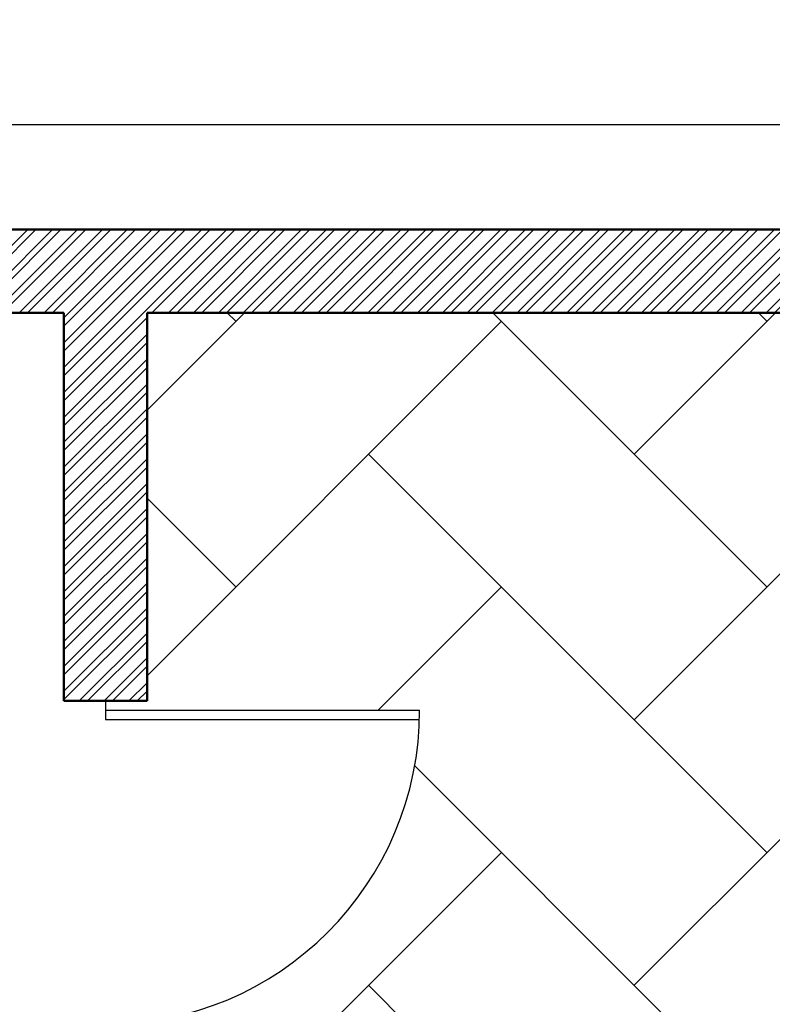
# Model space of a CAD drawing. Units: inches. Extents: x 3590 to 5167, y 65 to 1917.
# Tile 69 of 100: x 4919 to 5001, y 1722 to 1829. Entities that reach past the tile are written whole.
import ezdxf

# ---------------------------------------------------------------- set-up
doc = ezdxf.new("R2010")
doc.units = ezdxf.units.IN
for name, color, linetype, lineweight in [('A-ANNO-DIMS', 2, 'Continuous', 18), ('A-DOOR', 3, 'Continuous', 25), ('A-FLOR-PATT', 8, 'Continuous', 13), ('A-WALL', 7, 'Continuous', 50), ('A-WALL-PATT', 251, 'Continuous', 13)]:
    doc.layers.add(name, color=color, linetype=linetype, lineweight=lineweight)
doc.styles.get("Standard").update_dxf_attribs({"font": 'arial.ttf'})
doc.dimstyles.new('ISO-25', dxfattribs={"dimtxt": 9, "dimasz": 2.5, "dimexe": 1.25, "dimexo": 0.625, "dimtad": 1, "dimdec": 1, "dimlunit": 3, "dimtxsty": 'Standard', "dimcen": 2.5, "dimadec": 0, "dimazin": 0, "dimtfac": 1, "dimtdec": 1, "dimtmove": 0, "dimatfit": 3, "dimfxl": 1, "dimarcsym": 0})

# ---------------------------------------------------------------- blocks, each defined once
blk = doc.blocks.new('*D101')
at = {"layer": 'A-ANNO-DIMS', "color": 0, "lineweight": -2, "transparency": 16777216}
for p, q in [((4420.27, 1806.62), (4420.27, 1818.61)), ((5080.27, 1806.62), (5080.27, 1818.61)), ((4422.77, 1817.36), (5077.77, 1817.36))]:
    blk.add_line(p, q, dxfattribs=at)
at = {"layer": 'A-ANNO-DIMS', "color": 0, "transparency": 16777216}
for points in [[(4422.77, 1817.78), (4422.77, 1816.95), (4420.27, 1817.36)], [(5077.77, 1817.78), (5077.77, 1816.95), (5080.27, 1817.36)]]:
    blk.add_solid(points, dxfattribs=at)
at = {"layer": 'Defpoints', "color": 0, "transparency": 16777216}
for p in [(5080.27, 1817.36), (4420.27, 1806), (5080.27, 1806)]:
    blk.add_point(p, dxfattribs=at)
at = {"layer": 'A-ANNO-DIMS', "color": 0, "transparency": 16777216, "insert": (4750.27, 1822.57), "char_height": 9, "attachment_point": 5}
blk.add_mtext("55'", dxfattribs=at)
blk = doc.blocks.new('D1')
for p, q in [((1, 0), (1, 34)), ((2, 0), (2, 33.99)), ((0, 0), (2, 0)), ((35, 0), (36, 0))]:
    blk.add_line(p, q)
at = {"ltscale": 0.5}
blk.add_arc((1, 0), 34, 0, 90, dxfattribs=at)

msp = doc.modelspace()

# ---------------------------------------------------------------- hatches: boundary and pattern name
at = {"layer": 'A-FLOR-PATT', "transparency": 33554687}
h = msp.add_hatch(dxfattribs=at)
h.set_pattern_fill('AR-HBONE', color=256, scale=0.2)
h.set_pattern_definition([(45, (-588.972, 0), (0, 28.73682), [60.96, -20.32]), (135, (-574.604, 14.368), (3e-15, 28.73682), [60.96, -20.32])])
h.paths.add_polyline_path([(5071.27, 1797), (4933.27, 1797), (4933.27, 1754), (4962.77, 1754, -0.414214), (4928.77, 1720), (4933.27, 1719), (4933.27, 1335), (5071.27, 1335)])
h.paths.add_polyline_path([(4951.78, 1521.08), (4951.72, 1521.04), (4951.56, 1520.9)], flags=16)
h.paths.add_polyline_path([(4952.27, 1521.38), (4952.2, 1521.37), (4952.2, 1521.36)], flags=0)
h.paths.add_polyline_path([(4967.05, 1529.73), (4965.23, 1528.69), (4963.41, 1527.71), (4961.76, 1526.85), (4963.59, 1527.45), (4964.04, 1527.48), (4962.98, 1527.25), (4961.76, 1526.85), (4959.79, 1525.83), (4958, 1524.89), (4956.24, 1523.93), (4954.5, 1522.92), (4954.13, 1522.68), (4953.36, 1522), (4953.37, 1522), (4953.61, 1522.06), (4955.11, 1522.76), (4956.92, 1523.43), (4958.68, 1523.92), (4960.36, 1524.2), (4961.94, 1524.29), (4964.17, 1524.11), (4965.96, 1523.31), (4963.86, 1522.98), (4965.19, 1522.5), (4963.37, 1522.5), (4961.55, 1522.49), (4959.76, 1522.46), (4958.3, 1522.42), (4957.97, 1522.39), (4956.31, 1522.23), (4954.72, 1522.07), (4953.25, 1521.9), (4953.53, 1521.62), (4954.33, 1521.38), (4956.24, 1521.23), (4958.04, 1520.93), (4959.68, 1520.48), (4961.16, 1519.9), (4963.11, 1518.8), (4964.39, 1517.33), (4962.97, 1517.73), (4964.56, 1516.66), (4965.41, 1515.71), (4963.51, 1516.32), (4961.68, 1517.01), (4959.93, 1517.74), (4958.28, 1518.53), (4956.73, 1519.34), (4955.3, 1520.17), (4954.67, 1520.57), (4954.51, 1520.63), (4955.66, 1519.32), (4956.7, 1517.98), (4957.64, 1516.65), (4958.49, 1515.33), (4959.55, 1513.52), (4960.44, 1511.77), (4958.84, 1513.62), (4957.45, 1515.32), (4955.82, 1517.46), (4956.67, 1515.45), (4957.11, 1513.92), (4957.45, 1511.71), (4957.08, 1509.79), (4956.54, 1511.11), (4955.99, 1512.57), (4955.44, 1514.13), (4954.9, 1515.74), (4954.36, 1517.36), (4953.82, 1518.94), (4953.3, 1520.45), (4953.06, 1521.12), (4952.97, 1521.15), (4952.95, 1521.09), (4952.73, 1520.2), (4953.37, 1518.02), (4953.76, 1516.37), (4954.05, 1514.77), (4954.26, 1513.22), (4954.47, 1511.13), (4954.5, 1510.4), (4954.41, 1511.76), (4954.26, 1513.22), (4954.05, 1514.77), (4953.76, 1516.37), (4953.37, 1518.02), (4952.88, 1519.7), (4952.72, 1520.14), (4952.53, 1519.06), (4952.37, 1517.79), (4952.22, 1516.31), (4952.05, 1514.6), (4951.83, 1512.63), (4951.56, 1510.36), (4951.2, 1512.17), (4950.85, 1514.34), (4950.99, 1516.38), (4951.66, 1518.29), (4952.59, 1520.48), (4952.36, 1521.13), (4951.86, 1520.33), (4950.84, 1518.91), (4949.78, 1517.59), (4948.92, 1516.62), (4948.11, 1515.26), (4947.09, 1513.55), (4945.89, 1511.61), (4946.33, 1513.4), (4946.56, 1514.25), (4945.53, 1513.33), (4944.58, 1512.53), (4946.02, 1514.51), (4947.2, 1516.05), (4947.89, 1517.31), (4949.31, 1518.76), (4950.41, 1519.77), (4950.45, 1519.81), (4952.27, 1521.38), (4951.64, 1521.49), (4950.4, 1521.18), (4948.04, 1520.36), (4946.12, 1519.45), (4944.57, 1518.47), (4943.35, 1517.44), (4942, 1515.92), (4941.66, 1515.27), (4942.81, 1516.99), (4944.57, 1518.47), (4946.12, 1519.45), (4948.04, 1520.36), (4950.4, 1521.18), (4951.64, 1521.49), (4949.65, 1521.87), (4948.6, 1521.76), (4947.13, 1521.57), (4945.42, 1521.35), (4943.45, 1521.1), (4941.18, 1520.86), (4942.86, 1521.61), (4943.87, 1522.03), (4942.95, 1521.91), (4941.41, 1521.49), (4939.54, 1520.67), (4938.97, 1520.23), (4940.73, 1521.3), (4942.95, 1521.91), (4943.7, 1522.01), (4945.89, 1522.7), (4947.56, 1522.71), (4948.92, 1522.57), (4951.13, 1522.18), (4950.97, 1522.3), (4948.13, 1523.01), (4946.03, 1523.71), (4944.23, 1524.52), (4942.71, 1525.46), (4941.44, 1526.54), (4940.43, 1527.76), (4939.65, 1529.14), (4941.42, 1528.12), (4943.15, 1527.13), (4944.84, 1526.17), (4946.51, 1525.25), (4948.18, 1524.36), (4948.36, 1524.26), (4946.48, 1526.04), (4945.18, 1527.54), (4944.19, 1529.03), (4943.5, 1530.54), (4943.28, 1531.36), (4942.5, 1531.92), (4943.11, 1531.76), (4942.96, 1533.66), (4944.14, 1531.99), (4944.61, 1531.32), (4946.2, 1530.46), (4947.49, 1529.51), (4948.79, 1528.23), (4950.37, 1526.24), (4949.49, 1528.16), (4948.85, 1530.12), (4948.49, 1532.04), (4948.38, 1533.92), (4948.5, 1535.76), (4948.83, 1537.57), (4949.42, 1535.57), (4949.96, 1533.57), (4950.46, 1531.59), (4950.96, 1529.62), (4951.39, 1527.95), (4951.72, 1530.69), (4952.2, 1532.58), (4952.89, 1534.33), (4953.77, 1535.95), (4954.83, 1537.46), (4954.52, 1535.39), (4954.27, 1533.94), (4955.58, 1535.66), (4956.75, 1536.74), (4956.16, 1534.78), (4955.59, 1532.87), (4955.04, 1531.01), (4954.52, 1529.17), (4954.04, 1527.34), (4953.64, 1525.73), (4953.61, 1525.59), (4953.4, 1524.17), (4953.38, 1524.01), (4954.07, 1525.48), (4954.91, 1527.02), (4956.14, 1528.89), (4957.85, 1530.58), (4959.38, 1531.54), (4958.26, 1530.1), (4957.14, 1528.66), (4956.07, 1527.24), (4955.06, 1525.87), (4954.14, 1524.57), (4953.35, 1523.37), (4953.31, 1523.3), (4953.27, 1522.92), (4953.26, 1522.38), (4954.1, 1523.37), (4954.63, 1524.28), (4955.96, 1526.36), (4957.23, 1528.13), (4958.42, 1529.61), (4960.04, 1531.37), (4961.37, 1532.38), (4962.1, 1532.77), (4961.07, 1531.06), (4959.99, 1529.44), (4958.87, 1527.91), (4958.15, 1527.01), (4959.8, 1528), (4961.59, 1528.79), (4963.39, 1529.33), (4965.21, 1529.63)], flags=16)
h.paths.add_polyline_path([(4962.94, 1523.18), (4961.11, 1523.42), (4960.39, 1523.36), (4962.35, 1523.33)], flags=0)
h.paths.add_polyline_path([(5049.54, 1584.55), (5049.48, 1584.51), (5049.32, 1584.37)], flags=16)
h.paths.add_polyline_path([(5050.03, 1584.85), (5049.96, 1584.85), (5049.96, 1584.83)], flags=0)
h.paths.add_polyline_path([(5042.33, 1581.95), (5043.88, 1582.93), (5045.81, 1583.83), (5048.16, 1584.65), (5049.41, 1584.97), (5047.41, 1585.34), (5046.36, 1585.23), (5044.89, 1585.04), (5043.18, 1584.82), (5041.21, 1584.58), (5038.94, 1584.33), (5040.62, 1585.09), (5041.63, 1585.5), (5040.71, 1585.38), (5039.17, 1584.96), (5037.3, 1584.14), (5036.73, 1583.7), (5038.49, 1584.77), (5040.71, 1585.38), (5041.46, 1585.48), (5043.66, 1586.17), (5045.33, 1586.19), (5046.68, 1586.04), (5048.89, 1585.66), (5048.73, 1585.77), (5045.89, 1586.48), (5043.8, 1587.18), (5041.99, 1588), (5040.47, 1588.94), (5039.21, 1590.01), (5038.19, 1591.23), (5037.41, 1592.62), (5039.18, 1591.6), (5040.91, 1590.61), (5042.6, 1589.65), (5044.28, 1588.72), (5045.94, 1587.83), (5046.13, 1587.74), (5044.24, 1589.52), (5042.94, 1591.01), (5041.95, 1592.51), (5041.26, 1594.01), (5041.04, 1594.83), (5040.26, 1595.39), (5040.87, 1595.24), (5040.72, 1597.13), (5041.9, 1595.46), (5042.37, 1594.8), (5043.96, 1593.94), (5045.25, 1592.98), (5046.55, 1591.7), (5048.13, 1589.71), (5047.25, 1591.63), (5046.61, 1593.6), (5046.25, 1595.52), (5046.14, 1597.39), (5046.26, 1599.23), (5046.59, 1601.05), (5047.18, 1599.04), (5047.72, 1597.04), (5048.23, 1595.06), (5048.72, 1593.09), (5049.15, 1591.43), (5049.48, 1594.16), (5049.96, 1596.05), (5050.65, 1597.8), (5051.53, 1599.43), (5052.59, 1600.93), (5052.28, 1598.86), (5052.03, 1597.41), (5053.34, 1599.14), (5054.51, 1600.21), (5053.92, 1598.25), (5053.35, 1596.35), (5052.8, 1594.48), (5052.29, 1592.64), (5051.8, 1590.82), (5051.4, 1589.21), (5051.37, 1589.06), (5051.16, 1587.64), (5051.14, 1587.48), (5051.83, 1588.95), (5052.67, 1590.5), (5053.9, 1592.37), (5055.61, 1594.05), (5057.14, 1595.01), (5056.02, 1593.58), (5054.9, 1592.14), (5053.83, 1590.72), (5052.82, 1589.34), (5051.9, 1588.05), (5051.11, 1586.85), (5051.07, 1586.78), (5051.03, 1586.4), (5051.02, 1585.86), (5051.86, 1586.85), (5052.39, 1587.76), (5053.72, 1589.83), (5054.99, 1591.6), (5056.18, 1593.08), (5057.8, 1594.84), (5059.13, 1595.85), (5059.86, 1596.24), (5058.83, 1594.54), (5057.75, 1592.91), (5056.63, 1591.38), (5055.91, 1590.48), (5057.56, 1591.48), (5059.35, 1592.27), (5061.15, 1592.8), (5062.97, 1593.11), (5064.81, 1593.2), (5062.99, 1592.17), (5061.17, 1591.19), (5059.52, 1590.32), (5061.35, 1590.92), (5061.8, 1590.95), (5060.74, 1590.72), (5059.52, 1590.33), (5057.55, 1589.31), (5055.77, 1588.37), (5054, 1587.4), (5052.27, 1586.39), (5051.89, 1586.16), (5051.12, 1585.47), (5051.13, 1585.47), (5051.37, 1585.54), (5052.87, 1586.24), (5054.68, 1586.91), (5056.44, 1587.39), (5058.12, 1587.67), (5059.71, 1587.76), (5061.93, 1587.58), (5063.72, 1586.78), (5061.62, 1586.45), (5062.95, 1585.97), (5061.13, 1585.97), (5059.31, 1585.96), (5057.52, 1585.93), (5056.07, 1585.89), (5055.73, 1585.86), (5054.07, 1585.71), (5052.48, 1585.55), (5051.01, 1585.37), (5051.29, 1585.1), (5052.09, 1584.85), (5054, 1584.7), (5055.8, 1584.4), (5057.45, 1583.96), (5058.92, 1583.37), (5060.87, 1582.27), (5062.15, 1580.8), (5060.73, 1581.2), (5062.32, 1580.13), (5063.17, 1579.18), (5061.27, 1579.8), (5059.44, 1580.48), (5057.7, 1581.22), (5056.04, 1582), (5054.49, 1582.82), (5053.06, 1583.65), (5052.43, 1584.05), (5052.27, 1584.1), (5053.42, 1582.79), (5054.46, 1581.46), (5055.41, 1580.12), (5056.25, 1578.81), (5057.31, 1577), (5058.2, 1575.24), (5056.6, 1577.09), (5055.21, 1578.8), (5053.58, 1580.93), (5054.43, 1578.92), (5054.87, 1577.4), (5055.21, 1575.19), (5054.84, 1573.27), (5054.3, 1574.58), (5053.75, 1576.04), (5053.21, 1577.6), (5052.66, 1579.21), (5052.12, 1580.83), (5051.59, 1582.42), (5051.07, 1583.93), (5050.83, 1584.59), (5050.73, 1584.62), (5050.71, 1584.56), (5050.49, 1583.67), (5051.13, 1581.5), (5051.52, 1579.85), (5051.81, 1578.24), (5052.03, 1576.7), (5052.23, 1574.61), (5052.26, 1573.88), (5052.17, 1575.23), (5052.03, 1576.7), (5051.81, 1578.24), (5051.52, 1579.85), (5051.13, 1581.5), (5050.64, 1583.17), (5050.48, 1583.62), (5050.29, 1582.53), (5050.14, 1581.26), (5049.98, 1579.79), (5049.81, 1578.07), (5049.59, 1576.1), (5049.32, 1573.84), (5048.96, 1575.64), (5048.61, 1577.81), (5048.75, 1579.85), (5049.42, 1581.76), (5050.35, 1583.96), (5050.12, 1584.6), (5049.62, 1583.8), (5048.6, 1582.38), (5047.54, 1581.06), (5046.68, 1580.09), (5045.87, 1578.73), (5044.85, 1577.03), (5043.65, 1575.09), (5044.09, 1576.88), (5044.32, 1577.72), (5043.29, 1576.8), (5042.34, 1576.01), (5043.78, 1577.98), (5044.97, 1579.52), (5045.65, 1580.79), (5047.07, 1582.24), (5048.18, 1583.24), (5048.21, 1583.28), (5050.03, 1584.85), (5049.41, 1584.97), (5048.16, 1584.65), (5045.81, 1583.83), (5043.88, 1582.93), (5042.33, 1581.95), (5041.11, 1580.92), (5039.76, 1579.39), (5039.42, 1578.75), (5040.57, 1580.46)], flags=16)
h.paths.add_polyline_path([(4954.8, 1533.12), (4954.26, 1532.08), (4953.83, 1530.93), (4953.5, 1529.64), (4953.28, 1528.13), (4953.17, 1526.38), (4953.16, 1524.32), (4953.28, 1521.24), (4952.8, 1521.84), (4951.56, 1522), (4950.98, 1521.96), (4952.66, 1521.94), (4952.8, 1521.84), (4953.15, 1523.59), (4953.17, 1526.38), (4953.28, 1528.13), (4953.61, 1530.35), (4954.46, 1532.59)], flags=0)
h.paths.add_polyline_path([(5050.56, 1585.32), (5049.32, 1585.47), (5048.74, 1585.44), (5050.42, 1585.42), (5050.56, 1585.32), (5050.91, 1587.07), (5050.93, 1589.85), (5051.04, 1591.61), (5051.37, 1593.82), (5052.22, 1596.07), (5052.56, 1596.59), (5052.02, 1595.55), (5051.59, 1594.41), (5051.27, 1593.11), (5051.04, 1591.61), (5050.93, 1589.85), (5050.92, 1587.79), (5051.04, 1584.71)], flags=0)
h.paths.add_polyline_path([(5058.15, 1586.84), (5060.11, 1586.8), (5060.71, 1586.66), (5058.87, 1586.9)], flags=0)
h.paths.add_polyline_path([(5049.54, 1430.94), (5049.48, 1430.9), (5049.32, 1430.75)], flags=16)
h.paths.add_polyline_path([(5050.03, 1431.24), (5049.96, 1431.23), (5049.96, 1431.21)], flags=0)
h.paths.add_polyline_path([(5046.59, 1447.43), (5047.18, 1445.42), (5047.72, 1443.43), (5048.23, 1441.45), (5048.72, 1439.48), (5049.15, 1437.81), (5049.48, 1440.55), (5049.96, 1442.44), (5050.65, 1444.19), (5051.53, 1445.81), (5052.59, 1447.32), (5052.28, 1445.25), (5052.03, 1443.8), (5053.34, 1445.52), (5054.51, 1446.6), (5053.92, 1444.64), (5053.35, 1442.73), (5052.8, 1440.87), (5052.29, 1439.03), (5051.8, 1437.2), (5051.4, 1435.59), (5051.37, 1435.45), (5051.16, 1434.03), (5051.14, 1433.87), (5051.83, 1435.34), (5052.67, 1436.88), (5053.9, 1438.75), (5055.61, 1440.44), (5057.14, 1441.4), (5056.02, 1439.96), (5054.9, 1438.52), (5053.83, 1437.1), (5052.82, 1435.73), (5051.9, 1434.43), (5051.11, 1433.23), (5051.07, 1433.16), (5051.03, 1432.78), (5051.02, 1432.24), (5051.86, 1433.23), (5052.39, 1434.14), (5053.72, 1436.22), (5054.99, 1437.99), (5056.18, 1439.47), (5057.8, 1441.23), (5059.13, 1442.23), (5059.86, 1442.63), (5058.83, 1440.92), (5057.75, 1439.3), (5056.63, 1437.77), (5055.91, 1436.87), (5057.56, 1437.86), (5059.35, 1438.65), (5061.15, 1439.19), (5062.97, 1439.49), (5064.81, 1439.59), (5062.99, 1438.55), (5061.17, 1437.57), (5059.52, 1436.71), (5061.35, 1437.31), (5061.8, 1437.34), (5060.74, 1437.11), (5059.52, 1436.71), (5057.55, 1435.69), (5055.77, 1434.75), (5054, 1433.79), (5052.27, 1432.78), (5051.89, 1432.54), (5051.12, 1431.86), (5051.13, 1431.86), (5051.37, 1431.92), (5052.87, 1432.62), (5054.68, 1433.29), (5056.44, 1433.77), (5058.12, 1434.06), (5059.71, 1434.15), (5061.93, 1433.97), (5063.72, 1433.17), (5061.62, 1432.84), (5062.95, 1432.36), (5061.13, 1432.36), (5059.31, 1432.35), (5057.52, 1432.32), (5056.07, 1432.28), (5055.73, 1432.25), (5054.07, 1432.09), (5052.48, 1431.93), (5051.01, 1431.76), (5051.29, 1431.48), (5052.09, 1431.24), (5054, 1431.09), (5055.8, 1430.79), (5057.45, 1430.34), (5058.92, 1429.76), (5060.87, 1428.66), (5062.15, 1427.18), (5060.73, 1427.59), (5062.32, 1426.52), (5063.17, 1425.57), (5061.27, 1426.18), (5059.44, 1426.86), (5057.7, 1427.6), (5056.04, 1428.39), (5054.49, 1429.2), (5053.06, 1430.03), (5052.43, 1430.43), (5052.27, 1430.49), (5053.42, 1429.18), (5054.46, 1427.84), (5055.41, 1426.51), (5056.25, 1425.19), (5057.31, 1423.38), (5058.2, 1421.63), (5056.6, 1423.48), (5055.21, 1425.18), (5053.58, 1427.32), (5054.43, 1425.31), (5054.87, 1423.78), (5055.21, 1421.57), (5054.84, 1419.65), (5054.3, 1420.97), (5053.75, 1422.43), (5053.21, 1423.98), (5052.66, 1425.59), (5052.12, 1427.21), (5051.59, 1428.8), (5051.07, 1430.31), (5050.83, 1430.98), (5050.73, 1431.01), (5050.71, 1430.95), (5050.49, 1430.06), (5051.13, 1427.88), (5051.52, 1426.23), (5051.81, 1424.62), (5052.03, 1423.08), (5052.23, 1420.99), (5052.26, 1420.26), (5052.17, 1421.62), (5052.03, 1423.08), (5051.81, 1424.62), (5051.52, 1426.23), (5051.13, 1427.88), (5050.64, 1429.56), (5050.48, 1430), (5050.29, 1428.92), (5050.14, 1427.65), (5049.98, 1426.17), (5049.81, 1424.46), (5049.59, 1422.49), (5049.32, 1420.22), (5048.96, 1422.03), (5048.61, 1424.2), (5048.75, 1426.24), (5049.42, 1428.15), (5050.35, 1430.34), (5050.12, 1430.99), (5049.62, 1430.19), (5048.6, 1428.77), (5047.54, 1427.45), (5046.68, 1426.48), (5045.87, 1425.12), (5044.85, 1423.41), (5043.65, 1421.47), (5044.09, 1423.26), (5044.32, 1424.11), (5043.29, 1423.19), (5042.34, 1422.39), (5043.78, 1424.37), (5044.97, 1425.91), (5045.65, 1427.17), (5047.07, 1428.62), (5048.18, 1429.63), (5048.21, 1429.67), (5050.03, 1431.24), (5049.41, 1431.35), (5048.16, 1431.04), (5045.81, 1430.22), (5043.88, 1429.31), (5042.33, 1428.33), (5041.11, 1427.3), (5039.76, 1425.78), (5039.42, 1425.13), (5040.57, 1426.85), (5042.33, 1428.33), (5043.88, 1429.31), (5045.81, 1430.22), (5048.16, 1431.04), (5049.41, 1431.35), (5047.41, 1431.73), (5046.36, 1431.62), (5044.89, 1431.43), (5043.18, 1431.21), (5041.21, 1430.96), (5038.94, 1430.72), (5040.62, 1431.47), (5041.63, 1431.89), (5040.71, 1431.77), (5039.17, 1431.34), (5037.3, 1430.53), (5036.73, 1430.08), (5038.49, 1431.16), (5040.71, 1431.77), (5041.46, 1431.87), (5043.66, 1432.56), (5045.33, 1432.57), (5046.68, 1432.43), (5048.89, 1432.04), (5048.73, 1432.16), (5045.89, 1432.87), (5043.8, 1433.57), (5041.99, 1434.38), (5040.47, 1435.32), (5039.21, 1436.4), (5038.19, 1437.62), (5037.41, 1439), (5039.18, 1437.98), (5040.91, 1436.99), (5042.6, 1436.03), (5044.28, 1435.11), (5045.94, 1434.22), (5046.13, 1434.12), (5044.24, 1435.9), (5042.94, 1437.4), (5041.95, 1438.89), (5041.26, 1440.4), (5041.04, 1441.22), (5040.26, 1441.78), (5040.87, 1441.62), (5040.72, 1443.52), (5041.9, 1441.85), (5042.37, 1441.18), (5043.96, 1440.32), (5045.25, 1439.37), (5046.55, 1438.09), (5048.13, 1436.1), (5047.25, 1438.01), (5046.61, 1439.98), (5046.25, 1441.9), (5046.14, 1443.78), (5046.26, 1445.62)], flags=16)
h.paths.add_polyline_path([(5052.38, 1444.25), (5051.62, 1442.78), (5052.02, 1441.94), (5052.56, 1442.98)], flags=0)
h.paths.add_polyline_path([(5050.56, 1431.7), (5049.32, 1431.86), (5048.74, 1431.82), (5050.42, 1431.8)], flags=0)
h.paths.add_polyline_path([(5058.15, 1433.22), (5060.11, 1433.19), (5060.71, 1433.04), (5058.87, 1433.28)], flags=0)
h.paths.add_polyline_path([(5049.54, 1352.29), (5049.48, 1352.25), (5049.32, 1352.1)], flags=16)
h.paths.add_polyline_path([(5050.03, 1352.59), (5049.96, 1352.58), (5049.96, 1352.56)], flags=0)
h.paths.add_polyline_path([(5046.59, 1368.78), (5047.18, 1366.77), (5047.72, 1364.78), (5048.23, 1362.79), (5048.72, 1360.83), (5049.15, 1359.16), (5049.48, 1361.9), (5049.96, 1363.79), (5050.65, 1365.54), (5051.53, 1367.16), (5052.59, 1368.67), (5052.28, 1366.6), (5052.03, 1365.15), (5053.34, 1366.87), (5054.51, 1367.95), (5053.92, 1365.99), (5053.35, 1364.08), (5052.8, 1362.21), (5052.29, 1360.37), (5051.8, 1358.55), (5051.4, 1356.94), (5051.37, 1356.79), (5051.16, 1355.37), (5051.14, 1355.22), (5051.83, 1356.68), (5052.67, 1358.23), (5053.9, 1360.1), (5055.61, 1361.79), (5057.14, 1362.75), (5056.02, 1361.31), (5054.9, 1359.87), (5053.83, 1358.45), (5052.82, 1357.08), (5051.9, 1355.78), (5051.11, 1354.58), (5051.07, 1354.51), (5051.03, 1354.13), (5051.02, 1353.59), (5051.86, 1354.58), (5052.39, 1355.49), (5053.72, 1357.57), (5054.99, 1359.34), (5056.18, 1360.82), (5057.8, 1362.58), (5059.13, 1363.58), (5059.86, 1363.98), (5058.83, 1362.27), (5057.75, 1360.65), (5056.63, 1359.12), (5055.91, 1358.22), (5057.56, 1359.21), (5059.35, 1360), (5061.15, 1360.54), (5062.97, 1360.84), (5064.81, 1360.94), (5062.99, 1359.9), (5061.17, 1358.92), (5059.52, 1358.06), (5061.35, 1358.66), (5061.8, 1358.69), (5060.74, 1358.46), (5059.52, 1358.06), (5057.55, 1357.04), (5055.77, 1356.1), (5054, 1355.14), (5052.27, 1354.13), (5051.89, 1353.89), (5051.12, 1353.21), (5051.13, 1353.21), (5051.37, 1353.27), (5052.87, 1353.97), (5054.68, 1354.64), (5056.44, 1355.12), (5058.12, 1355.41), (5059.71, 1355.49), (5061.93, 1355.32), (5063.72, 1354.52), (5061.62, 1354.18), (5062.95, 1353.71), (5061.13, 1353.71), (5059.31, 1353.7), (5057.52, 1353.67), (5056.07, 1353.63), (5055.73, 1353.6), (5054.07, 1353.44), (5052.48, 1353.28), (5051.01, 1353.11), (5051.29, 1352.83), (5052.09, 1352.59), (5054, 1352.44), (5055.8, 1352.14), (5057.45, 1351.69), (5058.92, 1351.1), (5060.87, 1350.01), (5062.15, 1348.53), (5060.73, 1348.93), (5062.32, 1347.87), (5063.17, 1346.92), (5061.27, 1347.53), (5059.44, 1348.21), (5057.7, 1348.95), (5056.04, 1349.74), (5054.49, 1350.55), (5053.06, 1351.38), (5052.43, 1351.78), (5052.27, 1351.84), (5053.42, 1350.53), (5054.46, 1349.19), (5055.41, 1347.86), (5056.25, 1346.54), (5057.31, 1344.73), (5058.2, 1342.98), (5056.6, 1344.83), (5055.21, 1346.53), (5053.58, 1348.67), (5054.43, 1346.66), (5054.87, 1345.13), (5055.21, 1342.92), (5054.84, 1341), (5054.3, 1342.32), (5053.75, 1343.78), (5053.21, 1345.33), (5052.66, 1346.94), (5052.12, 1348.56), (5051.59, 1350.15), (5051.07, 1351.66), (5050.83, 1352.32), (5050.73, 1352.35), (5050.71, 1352.3), (5050.49, 1351.41), (5051.13, 1349.23), (5051.52, 1347.58), (5051.81, 1345.97), (5052.03, 1344.43), (5052.23, 1342.34), (5052.26, 1341.61), (5052.17, 1342.97), (5052.03, 1344.43), (5051.81, 1345.97), (5051.52, 1347.58), (5051.13, 1349.23), (5050.64, 1350.91), (5050.48, 1351.35), (5050.29, 1350.27), (5050.14, 1349), (5049.98, 1347.52), (5049.81, 1345.81), (5049.59, 1343.83), (5049.32, 1341.57), (5048.96, 1343.38), (5048.61, 1345.55), (5048.75, 1347.58), (5049.42, 1349.49), (5050.35, 1351.69), (5050.12, 1352.34), (5049.62, 1351.54), (5048.6, 1350.12), (5047.54, 1348.8), (5046.68, 1347.83), (5045.87, 1346.46), (5044.85, 1344.76), (5043.65, 1342.82), (5044.09, 1344.61), (5044.32, 1345.46), (5043.29, 1344.54), (5042.34, 1343.74), (5043.78, 1345.72), (5044.97, 1347.26), (5045.65, 1348.52), (5047.07, 1349.97), (5048.18, 1350.98), (5048.21, 1351.01), (5050.03, 1352.59), (5049.41, 1352.7), (5048.16, 1352.39), (5045.81, 1351.57), (5043.88, 1350.66), (5042.33, 1349.68), (5041.11, 1348.65), (5039.76, 1347.13), (5039.42, 1346.48), (5040.57, 1348.2), (5042.33, 1349.68), (5043.88, 1350.66), (5045.81, 1351.57), (5048.16, 1352.39), (5049.41, 1352.7), (5047.41, 1353.08), (5046.36, 1352.96), (5044.89, 1352.78), (5043.18, 1352.56), (5041.21, 1352.31), (5038.94, 1352.06), (5040.62, 1352.82), (5041.63, 1353.24), (5040.71, 1353.12), (5039.17, 1352.69), (5037.3, 1351.88), (5036.73, 1351.43), (5038.49, 1352.51), (5040.71, 1353.12), (5041.46, 1353.22), (5043.66, 1353.91), (5045.33, 1353.92), (5046.68, 1353.77), (5048.89, 1353.39), (5048.73, 1353.51), (5045.89, 1354.21), (5043.8, 1354.92), (5041.99, 1355.73), (5040.47, 1356.67), (5039.21, 1357.75), (5038.19, 1358.97), (5037.41, 1360.35), (5039.18, 1359.33), (5040.91, 1358.34), (5042.6, 1357.38), (5044.28, 1356.46), (5045.94, 1355.57), (5046.13, 1355.47), (5044.24, 1357.25), (5042.94, 1358.75), (5041.95, 1360.24), (5041.26, 1361.75), (5041.04, 1362.57), (5040.26, 1363.13), (5040.87, 1362.97), (5040.72, 1364.87), (5041.9, 1363.2), (5042.37, 1362.53), (5043.96, 1361.67), (5045.25, 1360.72), (5046.55, 1359.44), (5048.13, 1357.45), (5047.25, 1359.36), (5046.61, 1361.33), (5046.25, 1363.25), (5046.14, 1365.13), (5046.26, 1366.97)], flags=16)
h.paths.add_polyline_path([(5052.38, 1365.6), (5051.62, 1364.13), (5052.02, 1363.29), (5052.56, 1364.33)], flags=0)
h.paths.add_polyline_path([(4951.78, 1698.04), (4951.72, 1698), (4951.56, 1697.86)], flags=16)
h.paths.add_polyline_path([(4952.27, 1698.34), (4952.2, 1698.34), (4952.2, 1698.32)], flags=0)
h.paths.add_polyline_path([(4957.08, 1686.76), (4956.54, 1688.07), (4955.99, 1689.53), (4955.44, 1691.09), (4954.9, 1692.7), (4954.36, 1694.32), (4953.82, 1695.91), (4953.3, 1697.42), (4953.06, 1698.08), (4952.97, 1698.11), (4952.95, 1698.05), (4952.73, 1697.16), (4953.37, 1694.99), (4953.76, 1693.34), (4954.05, 1691.73), (4954.26, 1690.19), (4954.47, 1688.1), (4954.5, 1687.37), (4954.41, 1688.72), (4954.26, 1690.19), (4954.05, 1691.73), (4953.76, 1693.34), (4953.37, 1694.99), (4952.88, 1696.66), (4952.72, 1697.11), (4952.53, 1696.02), (4952.37, 1694.75), (4952.22, 1693.28), (4952.05, 1691.56), (4951.83, 1689.59), (4951.56, 1687.33), (4951.2, 1689.13), (4950.85, 1691.3), (4950.99, 1693.34), (4951.66, 1695.25), (4952.59, 1697.44), (4952.36, 1698.09), (4951.86, 1697.29), (4950.84, 1695.87), (4949.78, 1694.55), (4948.92, 1693.58), (4948.11, 1692.22), (4947.09, 1690.52), (4945.89, 1688.58), (4946.33, 1690.37), (4946.56, 1691.21), (4945.53, 1690.29), (4944.58, 1689.5), (4946.02, 1691.47), (4947.2, 1693.01), (4947.89, 1694.28), (4949.31, 1695.73), (4950.41, 1696.73), (4950.45, 1696.77), (4952.27, 1698.34), (4951.64, 1698.46), (4950.4, 1698.14), (4948.04, 1697.32), (4946.12, 1696.42), (4944.57, 1695.44), (4943.35, 1694.41), (4942, 1692.88), (4941.66, 1692.24), (4942.81, 1693.95), (4944.57, 1695.44), (4946.12, 1696.42), (4948.04, 1697.32), (4950.4, 1698.14), (4951.64, 1698.46), (4949.65, 1698.83), (4948.6, 1698.72), (4947.13, 1698.53), (4945.42, 1698.31), (4943.45, 1698.07), (4941.18, 1697.82), (4942.86, 1698.58), (4943.87, 1698.99), (4942.95, 1698.87), (4941.41, 1698.45), (4939.54, 1697.63), (4938.97, 1697.19), (4940.73, 1698.26), (4942.95, 1698.87), (4943.7, 1698.97), (4945.89, 1699.66), (4947.56, 1699.68), (4948.92, 1699.53), (4951.13, 1699.15), (4950.97, 1699.26), (4948.13, 1699.97), (4946.03, 1700.67), (4944.23, 1701.49), (4942.71, 1702.43), (4941.44, 1703.5), (4940.43, 1704.72), (4939.65, 1706.11), (4941.42, 1705.09), (4943.15, 1704.1), (4944.84, 1703.14), (4946.51, 1702.21), (4948.18, 1701.32), (4948.36, 1701.23), (4946.48, 1703.01), (4945.18, 1704.5), (4944.19, 1706), (4943.5, 1707.5), (4943.28, 1708.32), (4942.5, 1708.88), (4943.11, 1708.73), (4942.96, 1710.62), (4944.14, 1708.95), (4944.61, 1708.29), (4946.2, 1707.43), (4947.49, 1706.47), (4948.79, 1705.19), (4950.37, 1703.2), (4949.49, 1705.12), (4948.85, 1707.09), (4948.49, 1709.01), (4948.38, 1710.88), (4948.5, 1712.72), (4948.83, 1714.54), (4949.42, 1712.53), (4949.96, 1710.53), (4950.46, 1708.55), (4950.96, 1706.58), (4951.39, 1704.92), (4951.72, 1707.65), (4952.2, 1709.54), (4952.89, 1711.29), (4953.77, 1712.92), (4954.83, 1714.42), (4954.52, 1712.35), (4954.27, 1710.9), (4955.58, 1712.63), (4956.75, 1713.7), (4956.16, 1711.74), (4955.59, 1709.84), (4955.04, 1707.97), (4954.52, 1706.13), (4954.04, 1704.31), (4953.64, 1702.7), (4953.61, 1702.55), (4953.4, 1701.13), (4953.38, 1700.97), (4954.07, 1702.44), (4954.91, 1703.99), (4956.14, 1705.86), (4957.85, 1707.54), (4959.38, 1708.5), (4958.26, 1707.07), (4957.14, 1705.63), (4956.07, 1704.21), (4955.06, 1702.83), (4954.14, 1701.54), (4953.35, 1700.34), (4953.31, 1700.27), (4953.27, 1699.89), (4953.26, 1699.35), (4954.1, 1700.34), (4954.63, 1701.25), (4955.96, 1703.32), (4957.23, 1705.09), (4958.42, 1706.57), (4960.04, 1708.33), (4961.37, 1709.34), (4962.1, 1709.73), (4961.07, 1708.03), (4959.99, 1706.4), (4958.87, 1704.87), (4958.15, 1703.97), (4959.8, 1704.97), (4961.59, 1705.76), (4963.39, 1706.29), (4965.21, 1706.6), (4967.05, 1706.69), (4965.23, 1705.66), (4963.41, 1704.68), (4961.76, 1703.81), (4963.59, 1704.41), (4964.04, 1704.44), (4962.98, 1704.21), (4961.76, 1703.82), (4959.79, 1702.8), (4958, 1701.86), (4956.24, 1700.89), (4954.5, 1699.88), (4954.13, 1699.65), (4953.36, 1698.96), (4953.37, 1698.96), (4953.61, 1699.03), (4955.11, 1699.72), (4956.92, 1700.4), (4958.68, 1700.88), (4960.36, 1701.16), (4961.94, 1701.25), (4964.17, 1701.07), (4965.96, 1700.27), (4963.86, 1699.94), (4965.19, 1699.46), (4963.37, 1699.46), (4961.55, 1699.45), (4959.76, 1699.42), (4958.3, 1699.38), (4957.97, 1699.35), (4956.31, 1699.2), (4954.72, 1699.04), (4953.25, 1698.86), (4953.53, 1698.59), (4954.33, 1698.34), (4956.24, 1698.19), (4958.04, 1697.89), (4959.68, 1697.45), (4961.16, 1696.86), (4963.11, 1695.76), (4964.39, 1694.29), (4962.97, 1694.69), (4964.56, 1693.62), (4965.41, 1692.67), (4963.51, 1693.29), (4961.68, 1693.97), (4959.93, 1694.71), (4958.28, 1695.49), (4956.73, 1696.31), (4955.3, 1697.14), (4954.67, 1697.54), (4954.51, 1697.59), (4955.66, 1696.28), (4956.7, 1694.95), (4957.64, 1693.61), (4958.49, 1692.3), (4959.55, 1690.49), (4960.44, 1688.73), (4958.84, 1690.58), (4957.45, 1692.29), (4955.82, 1694.42), (4956.67, 1692.41), (4957.11, 1690.89), (4957.45, 1688.68)], flags=16)
h.paths.add_polyline_path([(5050.56, 1353.05), (5049.32, 1353.21), (5048.74, 1353.17), (5050.42, 1353.15)], flags=0)
h.paths.add_polyline_path([(4951.78, 1351.49), (4951.72, 1351.45), (4951.56, 1351.3)], flags=16)
h.paths.add_polyline_path([(4952.27, 1351.79), (4952.2, 1351.78), (4952.2, 1351.76)], flags=0)
h.paths.add_polyline_path([(4954.83, 1367.87), (4954.52, 1365.8), (4954.27, 1364.35), (4955.58, 1366.07), (4956.75, 1367.15), (4956.16, 1365.19), (4955.59, 1363.28), (4955.04, 1361.42), (4954.52, 1359.58), (4954.04, 1357.75), (4953.64, 1356.14), (4953.61, 1356), (4953.4, 1354.58), (4953.38, 1354.42), (4954.07, 1355.89), (4954.91, 1357.43), (4956.14, 1359.3), (4957.85, 1360.99), (4959.38, 1361.95), (4958.26, 1360.51), (4957.14, 1359.07), (4956.07, 1357.65), (4955.06, 1356.28), (4954.14, 1354.98), (4953.35, 1353.78), (4953.31, 1353.71), (4953.27, 1353.33), (4953.26, 1352.79), (4954.1, 1353.78), (4954.63, 1354.69), (4955.96, 1356.77), (4957.23, 1358.54), (4958.42, 1360.02), (4960.04, 1361.78), (4961.37, 1362.78), (4962.1, 1363.18), (4961.07, 1361.47), (4959.99, 1359.85), (4958.87, 1358.32), (4958.15, 1357.42), (4959.8, 1358.41), (4961.59, 1359.2), (4963.39, 1359.74), (4965.21, 1360.04), (4967.05, 1360.14), (4965.23, 1359.1), (4963.41, 1358.12), (4961.76, 1357.26), (4963.59, 1357.86), (4964.04, 1357.89), (4962.98, 1357.66), (4961.76, 1357.26), (4959.79, 1356.24), (4958, 1355.3), (4956.24, 1354.34), (4954.5, 1353.33), (4954.13, 1353.09), (4953.36, 1352.41), (4953.37, 1352.41), (4953.61, 1352.47), (4955.11, 1353.17), (4956.92, 1353.84), (4958.68, 1354.32), (4960.36, 1354.61), (4961.94, 1354.7), (4964.17, 1354.52), (4965.96, 1353.72), (4963.86, 1353.39), (4965.19, 1352.91), (4963.37, 1352.91), (4961.55, 1352.9), (4959.76, 1352.87), (4958.3, 1352.83), (4957.97, 1352.8), (4956.31, 1352.64), (4954.72, 1352.48), (4953.25, 1352.31), (4953.53, 1352.03), (4954.33, 1351.79), (4956.24, 1351.64), (4958.04, 1351.34), (4959.68, 1350.89), (4961.16, 1350.31), (4963.11, 1349.21), (4964.39, 1347.73), (4962.97, 1348.14), (4964.56, 1347.07), (4965.41, 1346.12), (4963.51, 1346.73), (4961.68, 1347.41), (4959.93, 1348.15), (4958.28, 1348.94), (4956.73, 1349.75), (4955.3, 1350.58), (4954.67, 1350.98), (4954.51, 1351.04), (4955.66, 1349.73), (4956.7, 1348.39), (4957.64, 1347.06), (4958.49, 1345.74), (4959.55, 1343.93), (4960.44, 1342.18), (4958.84, 1344.03), (4957.45, 1345.73), (4955.82, 1347.87), (4956.67, 1345.86), (4957.11, 1344.33), (4957.45, 1342.12), (4957.08, 1340.2), (4956.54, 1341.52), (4955.99, 1342.98), (4955.44, 1344.53), (4954.9, 1346.14), (4954.36, 1347.76), (4953.82, 1349.35), (4953.3, 1350.86), (4953.06, 1351.53), (4952.97, 1351.56), (4952.95, 1351.5), (4952.73, 1350.61), (4953.37, 1348.43), (4953.76, 1346.78), (4954.05, 1345.17), (4954.26, 1343.63), (4954.47, 1341.54), (4954.5, 1340.81), (4954.41, 1342.17), (4954.26, 1343.63), (4954.05, 1345.17), (4953.76, 1346.78), (4953.37, 1348.43), (4952.88, 1350.11), (4952.72, 1350.55), (4952.53, 1349.47), (4952.37, 1348.2), (4952.22, 1346.72), (4952.05, 1345.01), (4951.83, 1343.04), (4951.56, 1340.77), (4951.2, 1342.58), (4950.85, 1344.75), (4950.99, 1346.79), (4951.66, 1348.7), (4952.59, 1350.89), (4952.36, 1351.54), (4951.86, 1350.74), (4950.84, 1349.32), (4949.78, 1348), (4948.92, 1347.03), (4948.11, 1345.67), (4947.09, 1343.96), (4945.89, 1342.02), (4946.33, 1343.81), (4946.56, 1344.66), (4945.53, 1343.74), (4944.58, 1342.94), (4946.02, 1344.92), (4947.2, 1346.46), (4947.89, 1347.72), (4949.31, 1349.17), (4950.41, 1350.18), (4950.45, 1350.22), (4952.27, 1351.79), (4951.64, 1351.9), (4950.4, 1351.59), (4948.04, 1350.77), (4946.12, 1349.86), (4944.57, 1348.88), (4943.35, 1347.85), (4942, 1346.33), (4941.66, 1345.68), (4942.81, 1347.4), (4944.57, 1348.88), (4946.12, 1349.86), (4948.04, 1350.77), (4950.4, 1351.59), (4951.64, 1351.9), (4949.65, 1352.28), (4948.6, 1352.17), (4947.13, 1351.98), (4945.42, 1351.76), (4943.45, 1351.51), (4941.18, 1351.27), (4942.86, 1352.02), (4943.87, 1352.44), (4942.95, 1352.32), (4941.41, 1351.89), (4939.54, 1351.08), (4938.97, 1350.63), (4940.73, 1351.71), (4942.95, 1352.32), (4943.7, 1352.42), (4945.89, 1353.11), (4947.56, 1353.12), (4948.92, 1352.98), (4951.13, 1352.59), (4950.97, 1352.71), (4948.13, 1353.42), (4946.03, 1354.12), (4944.23, 1354.93), (4942.71, 1355.87), (4941.44, 1356.95), (4940.43, 1358.17), (4939.65, 1359.55), (4941.42, 1358.53), (4943.15, 1357.54), (4944.84, 1356.58), (4946.51, 1355.66), (4948.18, 1354.77), (4948.36, 1354.67), (4946.48, 1356.45), (4945.18, 1357.95), (4944.19, 1359.44), (4943.5, 1360.95), (4943.28, 1361.77), (4942.5, 1362.33), (4943.11, 1362.17), (4942.96, 1364.07), (4944.14, 1362.4), (4944.61, 1361.73), (4946.2, 1360.87), (4947.49, 1359.92), (4948.79, 1358.64), (4950.37, 1356.65), (4949.49, 1358.56), (4948.85, 1360.53), (4948.49, 1362.45), (4948.38, 1364.33), (4948.5, 1366.17), (4948.83, 1367.98), (4949.42, 1365.97), (4949.96, 1363.98), (4950.46, 1362), (4950.96, 1360.03), (4951.39, 1358.36), (4951.72, 1361.1), (4952.2, 1362.99), (4952.89, 1364.74), (4953.77, 1366.36)], flags=16)
h.paths.add_polyline_path([(4954.8, 1363.53), (4954.26, 1362.49), (4953.83, 1361.34), (4953.5, 1360.05), (4953.28, 1358.54), (4953.17, 1356.79), (4953.16, 1354.72), (4953.28, 1351.65), (4952.8, 1352.25), (4951.56, 1352.41), (4950.98, 1352.37), (4952.66, 1352.35), (4952.8, 1352.25), (4953.15, 1354), (4953.17, 1356.79), (4953.28, 1358.54), (4953.61, 1360.76), (4954.46, 1363)], flags=0)
h.paths.add_polyline_path([(4952.8, 1698.81), (4951.56, 1698.96), (4950.98, 1698.93), (4952.66, 1698.91), (4952.8, 1698.81), (4953.15, 1700.56), (4953.17, 1703.34), (4953.28, 1705.1), (4953.61, 1707.31), (4954.46, 1709.56), (4954.8, 1710.08), (4954.26, 1709.04), (4953.83, 1707.9), (4953.5, 1706.6), (4953.28, 1705.1), (4953.17, 1703.34), (4953.16, 1701.28), (4953.28, 1698.2)], flags=0)
h.paths.add_polyline_path([(4962.94, 1700.15), (4961.11, 1700.39), (4960.39, 1700.33), (4962.35, 1700.29)], flags=0)
h.paths.add_polyline_path([(5058.15, 1354.57), (5060.11, 1354.54), (5060.71, 1354.39), (5058.87, 1354.63)], flags=0)
h.paths.add_polyline_path([(4962.94, 1353.59), (4961.11, 1353.83), (4960.39, 1353.77), (4962.35, 1353.74)], flags=0)
h.paths.add_polyline_path([(5049.54, 1778.72), (5049.48, 1778.68), (5049.32, 1778.54)], flags=16)
h.paths.add_polyline_path([(5050.03, 1779.02), (5049.96, 1779.01), (5049.96, 1779)], flags=0)
h.paths.add_polyline_path([(5052.26, 1768.04), (5052.17, 1769.4), (5052.03, 1770.86), (5051.81, 1772.41), (5051.52, 1774.02), (5051.13, 1775.67), (5050.64, 1777.34), (5050.48, 1777.78), (5050.29, 1776.7), (5050.14, 1775.43), (5049.98, 1773.95), (5049.81, 1772.24), (5049.59, 1770.27), (5049.32, 1768.01), (5048.96, 1769.81), (5048.61, 1771.98), (5048.75, 1774.02), (5049.42, 1775.93), (5050.35, 1778.12), (5050.12, 1778.77), (5049.62, 1777.97), (5048.6, 1776.55), (5047.54, 1775.23), (5046.68, 1774.26), (5045.87, 1772.9), (5044.85, 1771.2), (5043.65, 1769.26), (5044.09, 1771.05), (5044.32, 1771.89), (5043.29, 1770.97), (5042.34, 1770.17), (5043.78, 1772.15), (5044.97, 1773.69), (5045.65, 1774.96), (5047.07, 1776.41), (5048.18, 1777.41), (5048.21, 1777.45), (5050.03, 1779.02), (5049.41, 1779.14), (5048.16, 1778.82), (5045.81, 1778), (5043.88, 1777.1), (5042.33, 1776.12), (5041.11, 1775.09), (5039.76, 1773.56), (5039.42, 1772.92), (5040.57, 1774.63), (5042.33, 1776.12), (5043.88, 1777.1), (5045.81, 1778), (5048.16, 1778.82), (5049.41, 1779.14), (5047.41, 1779.51), (5046.36, 1779.4), (5044.89, 1779.21), (5043.18, 1778.99), (5041.21, 1778.75), (5038.94, 1778.5), (5040.62, 1779.26), (5041.63, 1779.67), (5040.71, 1779.55), (5039.17, 1779.13), (5037.3, 1778.31), (5036.73, 1777.87), (5038.49, 1778.94), (5040.71, 1779.55), (5041.46, 1779.65), (5043.66, 1780.34), (5045.33, 1780.36), (5046.68, 1780.21), (5048.89, 1779.83), (5048.73, 1779.94), (5045.89, 1780.65), (5043.8, 1781.35), (5041.99, 1782.16), (5040.47, 1783.1), (5039.21, 1784.18), (5038.19, 1785.4), (5037.41, 1786.79), (5039.18, 1785.77), (5040.91, 1784.78), (5042.6, 1783.82), (5044.28, 1782.89), (5045.94, 1782), (5046.13, 1781.91), (5044.24, 1783.69), (5042.94, 1785.18), (5041.95, 1786.68), (5041.26, 1788.18), (5041.04, 1789), (5040.26, 1789.56), (5040.87, 1789.41), (5040.72, 1791.3), (5041.9, 1789.63), (5042.37, 1788.97), (5043.96, 1788.11), (5045.25, 1787.15), (5046.55, 1785.87), (5048.13, 1783.88), (5047.25, 1785.8), (5046.61, 1787.77), (5046.25, 1789.68), (5046.14, 1791.56), (5046.26, 1793.4), (5046.59, 1795.22), (5047.18, 1793.21), (5047.72, 1791.21), (5048.23, 1789.23), (5048.72, 1787.26), (5049.15, 1785.6), (5049.48, 1788.33), (5049.96, 1790.22), (5050.65, 1791.97), (5051.53, 1793.59), (5052.59, 1795.1), (5052.28, 1793.03), (5052.03, 1791.58), (5053.34, 1793.31), (5054.51, 1794.38), (5053.92, 1792.42), (5053.35, 1790.52), (5052.8, 1788.65), (5052.29, 1786.81), (5051.8, 1784.98), (5051.4, 1783.38), (5051.37, 1783.23), (5051.16, 1781.81), (5051.14, 1781.65), (5051.83, 1783.12), (5052.67, 1784.66), (5053.9, 1786.54), (5055.61, 1788.22), (5057.14, 1789.18), (5056.02, 1787.75), (5054.9, 1786.31), (5053.83, 1784.89), (5052.82, 1783.51), (5051.9, 1782.21), (5051.11, 1781.02), (5051.07, 1780.95), (5051.03, 1780.57), (5051.02, 1780.03), (5051.86, 1781.02), (5052.39, 1781.93), (5053.72, 1784), (5054.99, 1785.77), (5056.18, 1787.25), (5057.8, 1789.01), (5059.13, 1790.02), (5059.86, 1790.41), (5058.83, 1788.7), (5057.75, 1787.08), (5056.63, 1785.55), (5055.91, 1784.65), (5057.56, 1785.65), (5059.35, 1786.44), (5061.15, 1786.97), (5062.97, 1787.28), (5064.81, 1787.37), (5062.99, 1786.34), (5061.17, 1785.36), (5059.52, 1784.49), (5061.35, 1785.09), (5061.8, 1785.12), (5060.74, 1784.89), (5059.52, 1784.5), (5057.55, 1783.48), (5055.77, 1782.54), (5054, 1781.57), (5052.27, 1780.56), (5051.89, 1780.32), (5051.12, 1779.64), (5051.13, 1779.64), (5051.37, 1779.71), (5052.87, 1780.4), (5054.68, 1781.08), (5056.44, 1781.56), (5058.12, 1781.84), (5059.71, 1781.93), (5061.93, 1781.75), (5063.72, 1780.95), (5061.62, 1780.62), (5062.95, 1780.14), (5061.13, 1780.14), (5059.31, 1780.13), (5057.52, 1780.1), (5056.07, 1780.06), (5055.73, 1780.03), (5054.07, 1779.88), (5052.48, 1779.71), (5051.01, 1779.54), (5051.29, 1779.27), (5052.09, 1779.02), (5054, 1778.87), (5055.8, 1778.57), (5057.45, 1778.13), (5058.92, 1777.54), (5060.87, 1776.44), (5062.15, 1774.97), (5060.73, 1775.37), (5062.32, 1774.3), (5063.17, 1773.35), (5061.27, 1773.96), (5059.44, 1774.65), (5057.7, 1775.39), (5056.04, 1776.17), (5054.49, 1776.99), (5053.06, 1777.82), (5052.43, 1778.22), (5052.27, 1778.27), (5053.42, 1776.96), (5054.46, 1775.63), (5055.41, 1774.29), (5056.25, 1772.98), (5057.31, 1771.17), (5058.2, 1769.41), (5056.6, 1771.26), (5055.21, 1772.97), (5053.58, 1775.1), (5054.43, 1773.09), (5054.87, 1771.57), (5055.21, 1769.36), (5054.84, 1767.44), (5054.3, 1768.75), (5053.75, 1770.21), (5053.21, 1771.77), (5052.66, 1773.38), (5052.12, 1775), (5051.59, 1776.59), (5051.07, 1778.1), (5050.83, 1778.76), (5050.73, 1778.79), (5050.71, 1778.73), (5050.49, 1777.84), (5051.13, 1775.67), (5051.52, 1774.02), (5051.81, 1772.41), (5052.03, 1770.86), (5052.23, 1768.77)], flags=16)
h.paths.add_polyline_path([(5050.56, 1779.48), (5049.32, 1779.64), (5048.74, 1779.6), (5050.42, 1779.58), (5050.56, 1779.48), (5050.91, 1781.24), (5050.93, 1784.02), (5051.04, 1785.78), (5051.37, 1787.99), (5052.22, 1790.23), (5052.56, 1790.76), (5052.02, 1789.72), (5051.59, 1788.58), (5051.27, 1787.28), (5051.04, 1785.78), (5050.93, 1784.02), (5050.92, 1781.96), (5051.04, 1778.88)], flags=0)
h.paths.add_polyline_path([(5058.15, 1781), (5060.11, 1780.97), (5060.71, 1780.83), (5058.87, 1781.07)], flags=0)
at = {"layer": 'A-WALL-PATT', "transparency": 33554687}
h = msp.add_hatch(dxfattribs=at)
h.set_pattern_fill('ANSI32', color=256, scale=0.2)
h.paths.add_polyline_path([(4684.27, 1806), (4591.27, 1806), (4591.27, 1797), (4639.27, 1797), (4639.27, 1791), (4648.27, 1791), (4648.27, 1797), (4684.27, 1797)])
h.paths.add_polyline_path([(4543.27, 1806), (4420.27, 1806), (4420.27, 1785), (4429.27, 1785), (4429.27, 1797), (4445.92, 1797), (4543.27, 1797)])
h.paths.add_polyline_path([(4828.27, 1806), (4744.27, 1806), (4744.27, 1797), (4828.27, 1797)])
h.paths.add_polyline_path([(4648.27, 1755), (4639.27, 1755), (4639.27, 1656), (4546.27, 1656), (4546.27, 1650), (4549.27, 1650), (4549.27, 1554), (4429.27, 1554), (4429.27, 1584), (4420.27, 1584), (4420.27, 1539), (4429.27, 1539), (4429.27, 1545), (4639.27, 1545), (4639.27, 1539), (4648.27, 1539), (4648.27, 1560), (4639.27, 1560), (4639.27, 1554), (4555.27, 1554), (4555.27, 1650), (4639.27, 1650), (4639.27, 1590), (4648.27, 1590)])
h.paths.add_polyline_path([(4516.27, 1656), (4429.27, 1656), (4429.27, 1737), (4420.27, 1737), (4420.27, 1620), (4429.27, 1620), (4429.27, 1650), (4516.27, 1650)], flags=17)
h.paths.add_polyline_path([(5080.27, 1806), (4888.27, 1806), (4888.27, 1797), (4924.27, 1797), (4924.27, 1755), (4933.27, 1755), (4933.27, 1797), (5071.27, 1797), (5071.27, 1335), (4933.27, 1335), (4933.27, 1566), (4924.27, 1566), (4924.27, 1335), (4898.77, 1335), (4898.77, 1326), (5080.27, 1326)])
h.paths.add_polyline_path([(4933.27, 1719), (4924.27, 1719), (4924.27, 1638), (4933.27, 1638)], flags=17)
h.paths.add_polyline_path([(4802.77, 1335), (4777.27, 1335), (4777.27, 1503), (4756.27, 1503), (4756.27, 1494), (4768.27, 1494), (4768.27, 1431), (4696.27, 1431), (4696.27, 1494), (4708.27, 1494), (4708.27, 1503), (4639.27, 1503), (4639.27, 1494), (4687.27, 1494), (4687.27, 1431), (4681.27, 1431), (4681.27, 1422), (4768.27, 1422), (4768.27, 1335), (4726.27, 1335), (4726.27, 1326), (4802.77, 1326)])
h.paths.add_polyline_path([(4690.27, 1335), (4648.27, 1335), (4648.27, 1352.87), (4648.27, 1422), (4651.27, 1422), (4651.27, 1431), (4639.27, 1431), (4639.27, 1335), (4633.27, 1335), (4633.27, 1326), (4690.27, 1326)])
h.paths.add_polyline_path([(4585.27, 1335), (4584.72, 1335), (4429.27, 1335), (4429.27, 1491), (4420.27, 1491), (4420.27, 1326), (4585.27, 1326)])

# ---------------------------------------------------------------- linework, layer by layer
at = {"layer": 'A-WALL'}
for p, q in [((4648.27, 1797), (4924.27, 1797)), ((4924.27, 1755), (4924.27, 1797)), ((4933.27, 1797), (5071.27, 1797)), ((4933.27, 1755), (4933.27, 1797)), ((4924.27, 1755), (4933.27, 1755))]:
    msp.add_line(p, q, dxfattribs=at)
msp.add_lwpolyline([(5080.27, 1806), (5080.27, 1326), (4420.27, 1326), (4420.27, 1806)], close=True, dxfattribs=at)

# ---------------------------------------------------------------- block references
at = {"layer": 'A-DOOR', "rotation": 270}
msp.add_blockref('D1', (4928.77, 1755), dxfattribs=at)

# ---------------------------------------------------------------- dimensions: what is measured, and where the dimension line sits
at = {"layer": 'A-ANNO-DIMS'}
dim = msp.add_linear_dim(base=(5080.27, 1817.36), p1=(4420.27, 1806), p2=(5080.27, 1806), dimstyle='ISO-25', override={"dimclrd": 0, "dimclre": 0, "dimclrt": 0}, dxfattribs=at)
dim.commit()
dim.dimension.update_dxf_attribs({"geometry": '*D101', "text_midpoint": (4750.27, 1822.57)})

doc.saveas('drawing.dxf')
